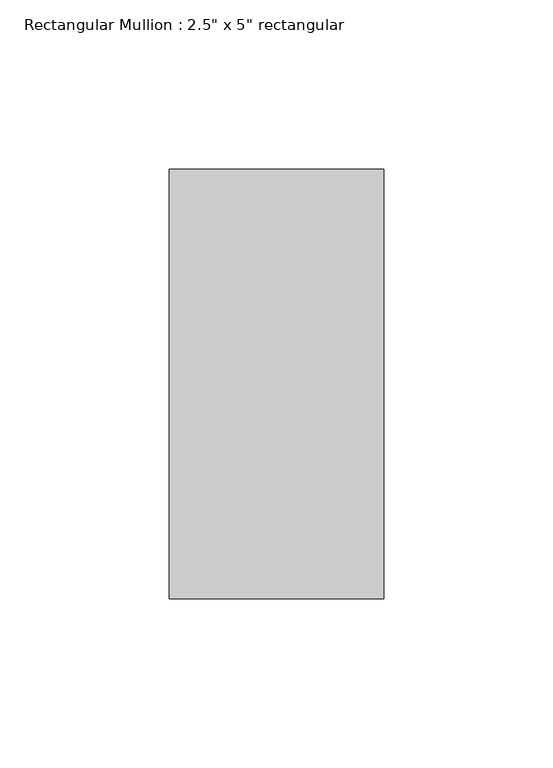
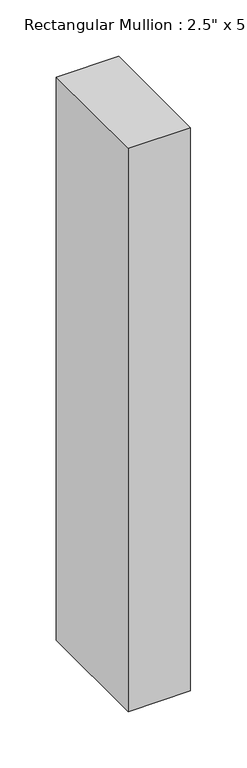
"""IFC4 building model written with IfcOpenShell, lengths in millimetres: member geometry."""

from ifc_helpers import new_model, si_unit, frame, origin, place, context, project, spatial, polyline, outline, extrude, source, transform, mapped, element, save


def member_a908bda9(model_context):
    return source(origin(), model_context, "Body", "SweptSolid", [
        extrude(outline(polyline([(0.0, 63.5), (0.0, -63.5), (-63.5, -63.5), (-63.5, 63.5), (0.0, 63.5)])), frame((0.0, 0.0, -609.1538352), z_axis=(0.0, 0.0, 1.0), x_axis=(1.0, 0.0, 0.0)), (0.0, 0.0, 1.0), 609.1538352),
    ])


if __name__ == "__main__":
    model = new_model("IFC4")
    model_context = context("Model", 3, world=origin())
    ifc_project = project(units=[si_unit("LENGTHUNIT", "METRE", prefix="MILLI")], contexts=[model_context])
    site = spatial("IfcSite", under=ifc_project)
    building = spatial("IfcBuilding", under=site)
    placement = place(None, origin())
    member_shape = member_a908bda9(model_context)
    element("IfcMember", 1, ObjectType="Rectangular Mullion : 2.5\" x 5\" rectangular", at=placement, inside=building, context=model_context, shape_type="MappedRepresentation", body=[
        mapped(member_shape, transform((0.0, 0.0, 0.0), x_axis=(1.0, 0.0, 0.0), y_axis=(0.0, 1.0, 0.0), z_axis=(0.0, 0.0, 1.0))),
    ])
    save(model, "model.ifc")

# Revit data of these elements
# Type "Rectangular Mullion : 2.5\" x 5\" rectangular"
#   built-in parameter 1007304 = 0.416667 (stored number, unit not read)
#   built-in parameter 1007301 = 0.104167 (stored number, unit not read)
#   built-in parameter 1007300 = 0.104167 (stored number, unit not read)
# Element 1 (IfcMember, "Rectangular Mullion : 2.5\" x 5\" rectangular")
#   Materials on its faces: "Aluminum"
# Materials
#   "Aluminum": class "Metal", colour RGB 247 247 247, transparency 0, Description = "Aluminum 6061", Cost = 0
